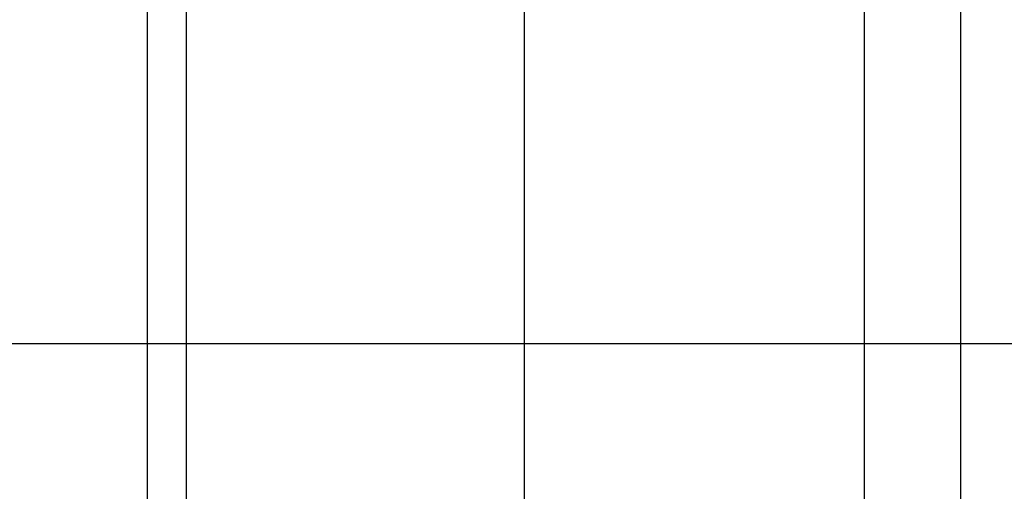
# Model space of a CAD drawing. Units: inches. Extents: x 2656 to 9931, y 1941 to 3068.
# Tile 7 of 46: x 2773 to 2811, y 2484 to 2502. Entities that reach past the tile are written whole.
import ezdxf

# ---------------------------------------------------------------- set-up
doc = ezdxf.new("R2010")
doc.units = ezdxf.units.IN
doc.layers.add('A-ANNO-DIMS', color=2, linetype='Continuous', lineweight=18)
doc.styles.get("Standard").update_dxf_attribs({"font": 'arial.ttf'})
doc.dimstyles.new('ISO-25', dxfattribs={"dimtxt": 6, "dimasz": 2.5, "dimexe": 1.25, "dimexo": 0.625, "dimtad": 1, "dimdec": 0, "dimlunit": 3, "dimtxsty": 'Standard', "dimcen": 2.5, "dimadec": 0, "dimazin": 0, "dimtfac": 1, "dimtdec": 0, "dimtmove": 0, "dimatfit": 3, "dimfxl": 1, "dimarcsym": 0})

# ---------------------------------------------------------------- blocks, each defined once
blk = doc.blocks.new('*D31')
at = {"layer": 'A-ANNO-DIMS', "color": 0, "lineweight": -2, "transparency": 16777216}
for p, q in [((2753.358, 2502.145), (2753.358, 2488.227)), ((2841.982, 2502.145), (2841.982, 2488.227)), ((2755.858, 2489.477), (2839.482, 2489.477)), ((2841.982, 2489.477), (2952.348, 2489.477))]:
    blk.add_line(p, q, dxfattribs=at)
at = {"layer": 'A-ANNO-DIMS', "color": 0, "transparency": 16777216}
for points in [[(2755.858, 2489.893), (2755.858, 2489.06), (2753.358, 2489.477)], [(2839.482, 2489.893), (2839.482, 2489.06), (2841.982, 2489.477)]]:
    blk.add_solid(points, dxfattribs=at)
at = {"layer": 'Defpoints', "color": 0, "transparency": 16777216}
for p in [(2753.358, 2502.77), (2841.982, 2502.77), (2841.982, 2489.477)]:
    blk.add_point(p, dxfattribs=at)
at = {"layer": 'A-ANNO-DIMS', "color": 0, "transparency": 16777216, "insert": (2898.415, 2493.206), "char_height": 6, "attachment_point": 5}
blk.add_mtext('DOUBLE BED 7\'-4 1/2" TYP.', dxfattribs=at)
blk = doc.blocks.new('*D113')
at = {"layer": 'A-ANNO-DIMS', "color": 0, "lineweight": -2, "transparency": 16777216}
for p, q in [((2752.157, 2300.725), (2752.157, 2674.45)), ((2809.769, 2300.725), (2809.769, 2674.45)), ((2754.657, 2673.2), (2807.269, 2673.2))]:
    blk.add_line(p, q, dxfattribs=at)
at = {"layer": 'A-ANNO-DIMS', "color": 0, "transparency": 16777216}
for points in [[(2754.657, 2673.617), (2754.657, 2672.784), (2752.157, 2673.2)], [(2807.269, 2673.617), (2807.269, 2672.784), (2809.769, 2673.2)]]:
    blk.add_solid(points, dxfattribs=at)
at = {"layer": 'Defpoints', "color": 0, "transparency": 16777216}
for p in [(2809.769, 2673.2), (2752.157, 2300.1), (2809.769, 2300.1)]:
    blk.add_point(p, dxfattribs=at)
at = {"layer": 'A-ANNO-DIMS', "color": 0, "transparency": 16777216, "insert": (2780.963, 2676.928), "char_height": 6, "attachment_point": 5}
blk.add_mtext('4\'-9 1/2"', dxfattribs=at)
blk = doc.blocks.new('*D114')
at = {"layer": 'A-ANNO-DIMS', "color": 0, "lineweight": -2, "transparency": 16777216}
for p, q in [((2809.769, 2300.725), (2809.769, 2674.45)), ((2851.877, 2300.725), (2851.877, 2674.45)), ((2812.269, 2673.2), (2849.377, 2673.2))]:
    blk.add_line(p, q, dxfattribs=at)
at = {"layer": 'A-ANNO-DIMS', "color": 0, "transparency": 16777216}
for points in [[(2812.269, 2673.617), (2812.269, 2672.784), (2809.769, 2673.2)], [(2849.377, 2673.617), (2849.377, 2672.784), (2851.877, 2673.2)]]:
    blk.add_solid(points, dxfattribs=at)
at = {"layer": 'Defpoints', "color": 0, "transparency": 16777216}
for p in [(2851.877, 2673.2), (2809.769, 2300.1), (2851.877, 2300.1)]:
    blk.add_point(p, dxfattribs=at)
at = {"layer": 'A-ANNO-DIMS', "color": 0, "transparency": 16777216, "insert": (2830.823, 2676.891), "char_height": 6, "attachment_point": 5}
blk.add_mtext('3\'-6"', dxfattribs=at)
blk = doc.blocks.new('*D129')
at = {"layer": 'A-ANNO-DIMS', "color": 0, "lineweight": -2, "transparency": 16777216}
for p, q in [((2752.157, 2601.146), (2752.157, 2009.273)), ((2777.587, 2557.74), (2777.587, 2009.273)), ((2754.657, 2010.523), (2775.087, 2010.523)), ((2777.587, 2010.523), (2811.37, 2010.523))]:
    blk.add_line(p, q, dxfattribs=at)
at = {"layer": 'A-ANNO-DIMS', "color": 0, "transparency": 16777216}
for points in [[(2754.657, 2010.939), (2754.657, 2010.106), (2752.157, 2010.523)], [(2775.087, 2010.939), (2775.087, 2010.106), (2777.587, 2010.523)]]:
    blk.add_solid(points, dxfattribs=at)
at = {"layer": 'Defpoints', "color": 0, "transparency": 16777216}
for p in [(2752.157, 2601.771), (2777.587, 2558.365), (2777.587, 2010.523)]:
    blk.add_point(p, dxfattribs=at)
at = {"layer": 'A-ANNO-DIMS', "color": 0, "transparency": 16777216, "insert": (2795.728, 2014.25), "char_height": 6, "attachment_point": 5}
blk.add_mtext('2\'-1 1/2"', dxfattribs=at)
blk = doc.blocks.new('*D132')
at = {"layer": 'A-ANNO-DIMS', "color": 0, "lineweight": -2, "transparency": 16777216}
for p, q in [((2763.467, 2366.557), (2763.467, 2674.45)), ((2805.965, 2366.557), (2805.965, 2674.45)), ((2765.967, 2673.2), (2803.465, 2673.2))]:
    blk.add_line(p, q, dxfattribs=at)
at = {"layer": 'A-ANNO-DIMS', "color": 0, "transparency": 16777216}
for points in [[(2765.967, 2673.617), (2765.967, 2672.784), (2763.467, 2673.2)], [(2803.465, 2673.617), (2803.465, 2672.784), (2805.965, 2673.2)]]:
    blk.add_solid(points, dxfattribs=at)
at = {"layer": 'Defpoints', "color": 0, "transparency": 16777216}
for p in [(2805.965, 2673.2), (2763.467, 2365.932), (2805.965, 2365.932)]:
    blk.add_point(p, dxfattribs=at)
at = {"layer": 'A-ANNO-DIMS', "color": 0, "transparency": 16777216, "insert": (2784.716, 2676.93), "char_height": 6, "attachment_point": 5}
blk.add_mtext('3\'-6 1/2"', dxfattribs=at)
blk = doc.blocks.new('*D134')
at = {"layer": 'A-ANNO-DIMS', "color": 0, "lineweight": -2, "transparency": 16777216}
for p, q in [((2752.157, 2300.725), (2752.157, 2674.45)), ((2763.467, 2347.433), (2763.467, 2674.45)), ((2754.657, 2673.2), (2760.967, 2673.2)), ((2763.467, 2673.2), (2801.809, 2673.2))]:
    blk.add_line(p, q, dxfattribs=at)
at = {"layer": 'A-ANNO-DIMS', "color": 0, "transparency": 16777216}
for points in [[(2754.657, 2673.617), (2754.657, 2672.784), (2752.157, 2673.2)], [(2760.967, 2673.617), (2760.967, 2672.784), (2763.467, 2673.2)]]:
    blk.add_solid(points, dxfattribs=at)
at = {"layer": 'Defpoints', "color": 0, "transparency": 16777216}
for p in [(2763.467, 2673.2), (2763.467, 2346.808), (2752.157, 2300.1)]:
    blk.add_point(p, dxfattribs=at)
at = {"layer": 'A-ANNO-DIMS', "color": 0, "transparency": 16777216, "insert": (2783.888, 2676.928), "char_height": 6, "attachment_point": 5}
blk.add_mtext('0\'-11 1/2"', dxfattribs=at)
blk = doc.blocks.new('*D136')
at = {"layer": 'A-ANNO-DIMS', "color": 0, "lineweight": -2, "transparency": 16777216}
for p, q in [((2765.357, 2375.042), (2765.357, 2674.45)), ((2779.142, 2375.042), (2779.142, 2674.45)), ((2767.857, 2673.2), (2776.642, 2673.2)), ((2779.142, 2673.2), (2798.277, 2673.2))]:
    blk.add_line(p, q, dxfattribs=at)
at = {"layer": 'A-ANNO-DIMS', "color": 0, "transparency": 16777216}
for points in [[(2767.857, 2673.617), (2767.857, 2672.784), (2765.357, 2673.2)], [(2776.642, 2673.617), (2776.642, 2672.784), (2779.142, 2673.2)]]:
    blk.add_solid(points, dxfattribs=at)
at = {"layer": 'Defpoints', "color": 0, "transparency": 16777216}
for p in [(2779.142, 2673.2), (2765.357, 2374.417), (2779.142, 2374.417)]:
    blk.add_point(p, dxfattribs=at)
at = {"layer": 'A-ANNO-DIMS', "color": 0, "transparency": 16777216, "insert": (2789.959, 2676.838), "char_height": 6, "attachment_point": 5}
blk.add_mtext('1\'-2"', dxfattribs=at)
blk = doc.blocks.new('*D137')
at = {"layer": 'A-ANNO-DIMS', "color": 0, "lineweight": -2, "transparency": 16777216}
for p, q in [((2779.142, 2375.042), (2779.142, 2674.45)), ((2792.516, 2375.042), (2792.516, 2674.45)), ((2781.642, 2673.2), (2790.016, 2673.2)), ((2792.516, 2673.2), (2825.632, 2673.2))]:
    blk.add_line(p, q, dxfattribs=at)
at = {"layer": 'A-ANNO-DIMS', "color": 0, "transparency": 16777216}
for points in [[(2781.642, 2673.617), (2781.642, 2672.784), (2779.142, 2673.2)], [(2790.016, 2673.617), (2790.016, 2672.784), (2792.516, 2673.2)]]:
    blk.add_solid(points, dxfattribs=at)
at = {"layer": 'Defpoints', "color": 0, "transparency": 16777216}
for p in [(2792.516, 2673.2), (2779.142, 2374.417), (2792.516, 2374.417)]:
    blk.add_point(p, dxfattribs=at)
at = {"layer": 'A-ANNO-DIMS', "color": 0, "transparency": 16777216, "insert": (2810.324, 2676.928), "char_height": 6, "attachment_point": 5}
blk.add_mtext('1\'-1 1/2"', dxfattribs=at)

msp = doc.modelspace()

# ---------------------------------------------------------------- dimensions: what is measured, and where the dimension line sits
at = {"layer": 'A-ANNO-DIMS'}
for base, p1, p2, picture, middle in [((2809.769, 2673.2), (2752.157, 2300.1), (2809.769, 2300.1), '*D113', (2780.963, 2676.928)), ((2763.467, 2673.2), (2752.157, 2300.1), (2763.467, 2346.808), '*D134', (2783.888, 2676.928)), ((2805.965, 2673.2), (2763.467, 2365.932), (2805.965, 2365.932), '*D132', (2784.716, 2676.93)), ((2792.516, 2673.2), (2779.142, 2374.417), (2792.516, 2374.417), '*D137', (2810.324, 2676.928)), ((2851.877, 2673.2), (2809.769, 2300.1), (2851.877, 2300.1), '*D114', (2830.823, 2676.891)), ((2779.142, 2673.2), (2765.357, 2374.417), (2779.142, 2374.417), '*D136', (2789.959, 2676.838)), ((2777.587, 2010.523), (2752.157, 2601.771), (2777.587, 2558.365), '*D129', (2795.728, 2014.25))]:
    dim = msp.add_linear_dim(base=base, p1=p1, p2=p2, dimstyle='ISO-25', override={"dimdec": 1, "dimlfac": 1, "dimrnd": 0, "dimzin": 1, "dimdsep": 46, "dimlunit": 4, "dimfrac": 2}, dxfattribs=at)
    dim.commit()
    dim.dimension.update_dxf_attribs({"geometry": picture, "text_midpoint": middle})
dim = msp.add_linear_dim(base=(2841.982, 2489.477), p1=(2753.358, 2502.77), p2=(2841.982, 2502.77), text='DOUBLE BED <> TYP.', dimstyle='ISO-25', override={"dimdec": 1, "dimlfac": 1, "dimrnd": 0, "dimzin": 1, "dimdsep": 46, "dimlunit": 4, "dimfrac": 2}, dxfattribs=at)
dim.commit()
dim.dimension.update_dxf_attribs({"geometry": '*D31', "text_midpoint": (2898.415, 2493.206)})

doc.saveas('drawing.dxf')
